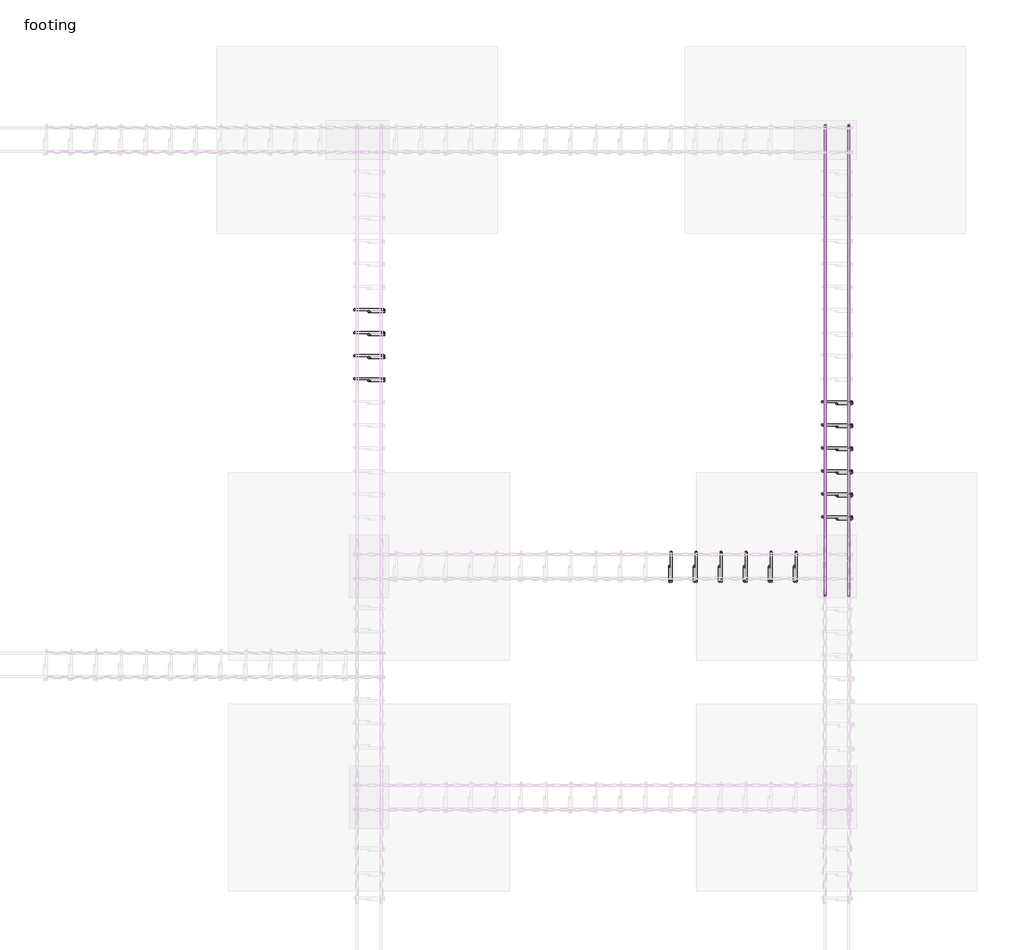
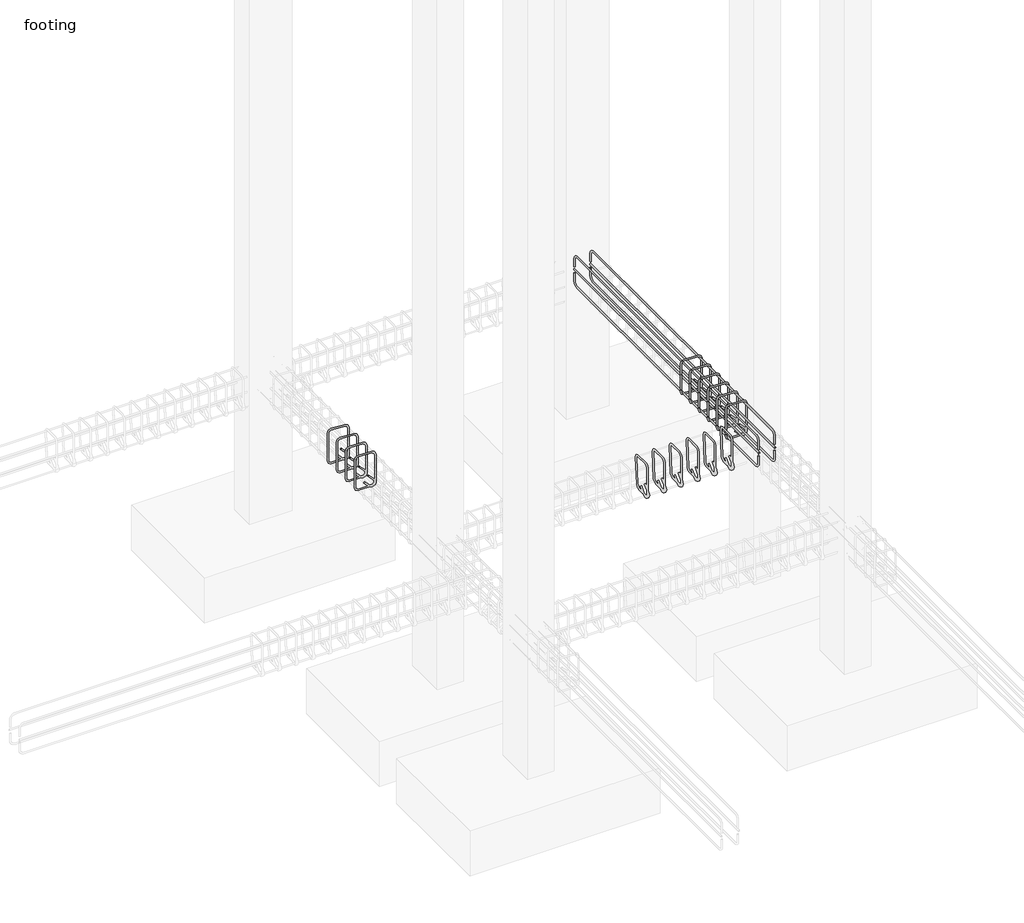
# One storey, part 19 of 21: 23 reinforcing bars.
"""IFC4 building model written with IfcOpenShell, lengths in millimetres."""

from ifc_helpers import new_model, si_unit, point, frame, origin, place, context, project, spatial, polyline, circle_curve, trimmed, segment, composite_curve, element, save
from ifc_brep_helpers import swept_disk

model = new_model("IFC4")

# Units and contexts
model_context = context("Model", 3, world=origin())
ifc_project = project(units=[si_unit("LENGTHUNIT", "METRE", prefix="MILLI")], contexts=[model_context])

# Site, building, storey
site = spatial("IfcSite", under=ifc_project)
building = spatial("IfcBuilding", under=site)
storey = spatial("IfcBuildingStorey", under=building, Name="footing", Elevation=-1524.0)

# Reinforcing bars
placement = place(None, origin())
element("IfcReinforcingBar", 1, at=placement, inside=storey, context=model_context, shape_type="SolidModel", body=[
    swept_disk(composite_curve([segment(polyline([(-5910.0883428, 8213.6387132, -310.8825168), (-5910.0883428, 8158.7737147, -365.7475153)]), True, "CONTINUOUS"), segment(trimmed(circle_curve(frame((-5910.0883428, 8136.3230744, -343.296875), z_axis=(-1.0, 0.0, 0.0), x_axis=(0.0, 22.450640299999577, -22.450640299999975)), 31.75), [point((-5910.0883428, 8158.7737147, -365.7475153))], [point((-5910.0883428, 8104.5730744, -343.296875))], True, "CARTESIAN"), True, "CONTINUOUS"), segment(polyline([(-5910.0883428, 8104.5730744, -343.296875), (-5910.0883428, 8104.5730744, -63.103125)]), True, "CONTINUOUS"), segment(trimmed(circle_curve(frame((-5910.0883428, 8136.3230744, -63.103125), z_axis=(-1.0, 0.0, 0.0), x_axis=(0.0, -31.75, 0.0)), 31.75), [point((-5910.0883428, 8104.5730744, -63.103125))], [point((-5910.0883428, 8136.3230744, -31.353125))], True, "CARTESIAN"), True, "CONTINUOUS"), segment(polyline([(-5910.0883428, 8136.3230744, -31.353125), (-5910.0883428, 8264.1168244, -31.353125)]), True, "CONTINUOUS"), segment(trimmed(circle_curve(frame((-5908.9159328, 8264.1168244, -63.0814712), z_axis=(-0.9993179916193466, 0.0, -0.03692629992126919), x_axis=(-1.1724100000001272, 0.0, 31.728346200000004)), 31.75), [point((-5910.0883428, 8264.1168244, -31.353125))], [point((-5908.9159328, 8295.8668244, -63.0814712))], True, "CARTESIAN"), True, "CONTINUOUS"), segment(polyline([(-5908.9159328, 8295.8668244, -63.0814712), (-5898.5607528, 8295.8668244, -343.3185288)]), True, "CONTINUOUS"), segment(trimmed(circle_curve(frame((-5898.5607528, 8264.1168244, -343.3185288), z_axis=(-0.9993179916193466, 0.0, -0.03692629992126919), x_axis=(0.0, 31.75, 0.0)), 31.75), [point((-5898.5607528, 8295.8668244, -343.3185288))], [point((-5897.3883428, 8264.1168244, -375.046875))], True, "CARTESIAN"), True, "CONTINUOUS"), segment(polyline([(-5897.3883428, 8264.1168244, -375.046875), (-5897.3883428, 8136.3230744, -375.046875)]), True, "CONTINUOUS"), segment(trimmed(circle_curve(frame((-5897.3883428, 8136.3230744, -343.296875), z_axis=(-1.0, 0.0, 0.0), x_axis=(0.0, 0.0, -31.75)), 31.75), [point((-5897.3883428, 8136.3230744, -375.046875))], [point((-5897.3883428, 8113.8724341, -320.8462347))], True, "CARTESIAN"), True, "CONTINUOUS"), segment(polyline([(-5897.3883428, 8113.8724341, -320.8462347), (-5897.3883428, 8168.7374326, -265.9812362)]), True, "CONTINUOUS")], self_intersect=False), 6.35),
])
element("IfcReinforcingBar", 2, at=placement, inside=storey, context=model_context, shape_type="SolidModel", body=[
    swept_disk(composite_curve([segment(polyline([(-5747.3883428, 8213.6387132, -310.8825168), (-5747.3883428, 8158.7737147, -365.7475153)]), True, "CONTINUOUS"), segment(trimmed(circle_curve(frame((-5747.3883428, 8136.3230744, -343.296875), z_axis=(-1.0, 0.0, 0.0), x_axis=(0.0, 22.450640299999577, -22.450640299999975)), 31.75), [point((-5747.3883428, 8158.7737147, -365.7475153))], [point((-5747.3883428, 8104.5730744, -343.296875))], True, "CARTESIAN"), True, "CONTINUOUS"), segment(polyline([(-5747.3883428, 8104.5730744, -343.296875), (-5747.3883428, 8104.5730744, -63.103125)]), True, "CONTINUOUS"), segment(trimmed(circle_curve(frame((-5747.3883428, 8136.3230744, -63.103125), z_axis=(-1.0, 0.0, 0.0), x_axis=(0.0, -31.75, 0.0)), 31.75), [point((-5747.3883428, 8104.5730744, -63.103125))], [point((-5747.3883428, 8136.3230744, -31.353125))], True, "CARTESIAN"), True, "CONTINUOUS"), segment(polyline([(-5747.3883428, 8136.3230744, -31.353125), (-5747.3883428, 8264.1168244, -31.353125)]), True, "CONTINUOUS"), segment(trimmed(circle_curve(frame((-5746.2159328, 8264.1168244, -63.0814712), z_axis=(-0.9993179916193466, 0.0, -0.03692629992126919), x_axis=(-1.1724100000001272, 0.0, 31.728346200000004)), 31.75), [point((-5747.3883428, 8264.1168244, -31.353125))], [point((-5746.2159328, 8295.8668244, -63.0814712))], True, "CARTESIAN"), True, "CONTINUOUS"), segment(polyline([(-5746.2159328, 8295.8668244, -63.0814712), (-5735.8607528, 8295.8668244, -343.3185288)]), True, "CONTINUOUS"), segment(trimmed(circle_curve(frame((-5735.8607528, 8264.1168244, -343.3185288), z_axis=(-0.9993179916193466, 0.0, -0.03692629992126919), x_axis=(0.0, 31.75, 0.0)), 31.75), [point((-5735.8607528, 8295.8668244, -343.3185288))], [point((-5734.6883428, 8264.1168244, -375.046875))], True, "CARTESIAN"), True, "CONTINUOUS"), segment(polyline([(-5734.6883428, 8264.1168244, -375.046875), (-5734.6883428, 8136.3230744, -375.046875)]), True, "CONTINUOUS"), segment(trimmed(circle_curve(frame((-5734.6883428, 8136.3230744, -343.296875), z_axis=(-1.0, 0.0, 0.0), x_axis=(0.0, 0.0, -31.75)), 31.75), [point((-5734.6883428, 8136.3230744, -375.046875))], [point((-5734.6883428, 8113.8724341, -320.8462347))], True, "CARTESIAN"), True, "CONTINUOUS"), segment(polyline([(-5734.6883428, 8113.8724341, -320.8462347), (-5734.6883428, 8168.7374326, -265.9812362)]), True, "CONTINUOUS")], self_intersect=False), 6.35),
])
element("IfcReinforcingBar", 3, at=placement, inside=storey, context=model_context, shape_type="SolidModel", body=[
    swept_disk(composite_curve([segment(polyline([(-5584.6883428, 8213.6387132, -310.8825168), (-5584.6883428, 8158.7737147, -365.7475153)]), True, "CONTINUOUS"), segment(trimmed(circle_curve(frame((-5584.6883428, 8136.3230744, -343.296875), z_axis=(-1.0, 0.0, 0.0), x_axis=(0.0, 22.450640299999577, -22.450640299999975)), 31.75), [point((-5584.6883428, 8158.7737147, -365.7475153))], [point((-5584.6883428, 8104.5730744, -343.296875))], True, "CARTESIAN"), True, "CONTINUOUS"), segment(polyline([(-5584.6883428, 8104.5730744, -343.296875), (-5584.6883428, 8104.5730744, -63.103125)]), True, "CONTINUOUS"), segment(trimmed(circle_curve(frame((-5584.6883428, 8136.3230744, -63.103125), z_axis=(-1.0, 0.0, 0.0), x_axis=(0.0, -31.75, 0.0)), 31.75), [point((-5584.6883428, 8104.5730744, -63.103125))], [point((-5584.6883428, 8136.3230744, -31.353125))], True, "CARTESIAN"), True, "CONTINUOUS"), segment(polyline([(-5584.6883428, 8136.3230744, -31.353125), (-5584.6883428, 8264.1168244, -31.353125)]), True, "CONTINUOUS"), segment(trimmed(circle_curve(frame((-5583.5159328, 8264.1168244, -63.0814712), z_axis=(-0.9993179916193466, 0.0, -0.03692629992126919), x_axis=(-1.1724100000001272, 0.0, 31.728346200000004)), 31.75), [point((-5584.6883428, 8264.1168244, -31.353125))], [point((-5583.5159328, 8295.8668244, -63.0814712))], True, "CARTESIAN"), True, "CONTINUOUS"), segment(polyline([(-5583.5159328, 8295.8668244, -63.0814712), (-5573.1607528, 8295.8668244, -343.3185288)]), True, "CONTINUOUS"), segment(trimmed(circle_curve(frame((-5573.1607528, 8264.1168244, -343.3185288), z_axis=(-0.9993179916193466, 0.0, -0.03692629992126919), x_axis=(0.0, 31.75, 0.0)), 31.75), [point((-5573.1607528, 8295.8668244, -343.3185288))], [point((-5571.9883428, 8264.1168244, -375.046875))], True, "CARTESIAN"), True, "CONTINUOUS"), segment(polyline([(-5571.9883428, 8264.1168244, -375.046875), (-5571.9883428, 8136.3230744, -375.046875)]), True, "CONTINUOUS"), segment(trimmed(circle_curve(frame((-5571.9883428, 8136.3230744, -343.296875), z_axis=(-1.0, 0.0, 0.0), x_axis=(0.0, 0.0, -31.75)), 31.75), [point((-5571.9883428, 8136.3230744, -375.046875))], [point((-5571.9883428, 8113.8724341, -320.8462347))], True, "CARTESIAN"), True, "CONTINUOUS"), segment(polyline([(-5571.9883428, 8113.8724341, -320.8462347), (-5571.9883428, 8168.7374326, -265.9812362)]), True, "CONTINUOUS")], self_intersect=False), 6.35),
])
element("IfcReinforcingBar", 4, at=placement, inside=storey, context=model_context, shape_type="SolidModel", body=[
    swept_disk(composite_curve([segment(polyline([(-5421.9883428, 8213.6387132, -310.8825168), (-5421.9883428, 8158.7737147, -365.7475153)]), True, "CONTINUOUS"), segment(trimmed(circle_curve(frame((-5421.9883428, 8136.3230744, -343.296875), z_axis=(-1.0, 0.0, 0.0), x_axis=(0.0, 22.450640299999577, -22.450640299999975)), 31.75), [point((-5421.9883428, 8158.7737147, -365.7475153))], [point((-5421.9883428, 8104.5730744, -343.296875))], True, "CARTESIAN"), True, "CONTINUOUS"), segment(polyline([(-5421.9883428, 8104.5730744, -343.296875), (-5421.9883428, 8104.5730744, -63.103125)]), True, "CONTINUOUS"), segment(trimmed(circle_curve(frame((-5421.9883428, 8136.3230744, -63.103125), z_axis=(-1.0, 0.0, 0.0), x_axis=(0.0, -31.75, 0.0)), 31.75), [point((-5421.9883428, 8104.5730744, -63.103125))], [point((-5421.9883428, 8136.3230744, -31.353125))], True, "CARTESIAN"), True, "CONTINUOUS"), segment(polyline([(-5421.9883428, 8136.3230744, -31.353125), (-5421.9883428, 8264.1168244, -31.353125)]), True, "CONTINUOUS"), segment(trimmed(circle_curve(frame((-5420.8159328, 8264.1168244, -63.0814712), z_axis=(-0.9993179916193466, 0.0, -0.03692629992126919), x_axis=(-1.1724100000001272, 0.0, 31.728346200000004)), 31.75), [point((-5421.9883428, 8264.1168244, -31.353125))], [point((-5420.8159328, 8295.8668244, -63.0814712))], True, "CARTESIAN"), True, "CONTINUOUS"), segment(polyline([(-5420.8159328, 8295.8668244, -63.0814712), (-5410.4607528, 8295.8668244, -343.3185288)]), True, "CONTINUOUS"), segment(trimmed(circle_curve(frame((-5410.4607528, 8264.1168244, -343.3185288), z_axis=(-0.9993179916193466, 0.0, -0.03692629992126919), x_axis=(0.0, 31.75, 0.0)), 31.75), [point((-5410.4607528, 8295.8668244, -343.3185288))], [point((-5409.2883428, 8264.1168244, -375.046875))], True, "CARTESIAN"), True, "CONTINUOUS"), segment(polyline([(-5409.2883428, 8264.1168244, -375.046875), (-5409.2883428, 8136.3230744, -375.046875)]), True, "CONTINUOUS"), segment(trimmed(circle_curve(frame((-5409.2883428, 8136.3230744, -343.296875), z_axis=(-1.0, 0.0, 0.0), x_axis=(0.0, 0.0, -31.75)), 31.75), [point((-5409.2883428, 8136.3230744, -375.046875))], [point((-5409.2883428, 8113.8724341, -320.8462347))], True, "CARTESIAN"), True, "CONTINUOUS"), segment(polyline([(-5409.2883428, 8113.8724341, -320.8462347), (-5409.2883428, 8168.7374326, -265.9812362)]), True, "CONTINUOUS")], self_intersect=False), 6.35),
])
element("IfcReinforcingBar", 5, at=placement, inside=storey, context=model_context, shape_type="SolidModel", body=[
    swept_disk(composite_curve([segment(polyline([(-5259.2883428, 8213.6387132, -310.8825168), (-5259.2883428, 8158.7737147, -365.7475153)]), True, "CONTINUOUS"), segment(trimmed(circle_curve(frame((-5259.2883428, 8136.3230744, -343.296875), z_axis=(-1.0, 0.0, 0.0), x_axis=(0.0, 22.450640299999577, -22.450640299999975)), 31.75), [point((-5259.2883428, 8158.7737147, -365.7475153))], [point((-5259.2883428, 8104.5730744, -343.296875))], True, "CARTESIAN"), True, "CONTINUOUS"), segment(polyline([(-5259.2883428, 8104.5730744, -343.296875), (-5259.2883428, 8104.5730744, -63.103125)]), True, "CONTINUOUS"), segment(trimmed(circle_curve(frame((-5259.2883428, 8136.3230744, -63.103125), z_axis=(-1.0, 0.0, 0.0), x_axis=(0.0, -31.75, 0.0)), 31.75), [point((-5259.2883428, 8104.5730744, -63.103125))], [point((-5259.2883428, 8136.3230744, -31.353125))], True, "CARTESIAN"), True, "CONTINUOUS"), segment(polyline([(-5259.2883428, 8136.3230744, -31.353125), (-5259.2883428, 8264.1168244, -31.353125)]), True, "CONTINUOUS"), segment(trimmed(circle_curve(frame((-5258.1159328, 8264.1168244, -63.0814712), z_axis=(-0.9993179916193466, 0.0, -0.03692629992126919), x_axis=(-1.1724099999992177, 0.0, 31.728346200000004)), 31.75), [point((-5259.2883428, 8264.1168244, -31.353125))], [point((-5258.1159328, 8295.8668244, -63.0814712))], True, "CARTESIAN"), True, "CONTINUOUS"), segment(polyline([(-5258.1159328, 8295.8668244, -63.0814712), (-5247.7607528, 8295.8668244, -343.3185288)]), True, "CONTINUOUS"), segment(trimmed(circle_curve(frame((-5247.7607528, 8264.1168244, -343.3185288), z_axis=(-0.9993179916193466, 0.0, -0.03692629992126919), x_axis=(0.0, 31.75, 0.0)), 31.75), [point((-5247.7607528, 8295.8668244, -343.3185288))], [point((-5246.5883428, 8264.1168244, -375.046875))], True, "CARTESIAN"), True, "CONTINUOUS"), segment(polyline([(-5246.5883428, 8264.1168244, -375.046875), (-5246.5883428, 8136.3230744, -375.046875)]), True, "CONTINUOUS"), segment(trimmed(circle_curve(frame((-5246.5883428, 8136.3230744, -343.296875), z_axis=(-1.0, 0.0, 0.0), x_axis=(0.0, 0.0, -31.75)), 31.75), [point((-5246.5883428, 8136.3230744, -375.046875))], [point((-5246.5883428, 8113.8724341, -320.8462347))], True, "CARTESIAN"), True, "CONTINUOUS"), segment(polyline([(-5246.5883428, 8113.8724341, -320.8462347), (-5246.5883428, 8168.7374326, -265.9812362)]), True, "CONTINUOUS")], self_intersect=False), 6.35),
])
element("IfcReinforcingBar", 6, at=placement, inside=storey, context=model_context, shape_type="SolidModel", body=[
    swept_disk(composite_curve([segment(polyline([(-5096.5883428, 8213.6387132, -310.8825168), (-5096.5883428, 8158.7737147, -365.7475153)]), True, "CONTINUOUS"), segment(trimmed(circle_curve(frame((-5096.5883428, 8136.3230744, -343.296875), z_axis=(-1.0, 0.0, 0.0), x_axis=(0.0, 22.450640299999577, -22.450640299999975)), 31.75), [point((-5096.5883428, 8158.7737147, -365.7475153))], [point((-5096.5883428, 8104.5730744, -343.296875))], True, "CARTESIAN"), True, "CONTINUOUS"), segment(polyline([(-5096.5883428, 8104.5730744, -343.296875), (-5096.5883428, 8104.5730744, -63.103125)]), True, "CONTINUOUS"), segment(trimmed(circle_curve(frame((-5096.5883428, 8136.3230744, -63.103125), z_axis=(-1.0, 0.0, 0.0), x_axis=(0.0, -31.75, 0.0)), 31.75), [point((-5096.5883428, 8104.5730744, -63.103125))], [point((-5096.5883428, 8136.3230744, -31.353125))], True, "CARTESIAN"), True, "CONTINUOUS"), segment(polyline([(-5096.5883428, 8136.3230744, -31.353125), (-5096.5883428, 8264.1168244, -31.353125)]), True, "CONTINUOUS"), segment(trimmed(circle_curve(frame((-5095.4159328, 8264.1168244, -63.0814712), z_axis=(-0.9993179916193466, 0.0, -0.03692629992126919), x_axis=(-1.1724100000001272, 0.0, 31.728346200000004)), 31.75), [point((-5096.5883428, 8264.1168244, -31.353125))], [point((-5095.4159328, 8295.8668244, -63.0814712))], True, "CARTESIAN"), True, "CONTINUOUS"), segment(polyline([(-5095.4159328, 8295.8668244, -63.0814712), (-5085.0607528, 8295.8668244, -343.3185288)]), True, "CONTINUOUS"), segment(trimmed(circle_curve(frame((-5085.0607528, 8264.1168244, -343.3185288), z_axis=(-0.9993179916193466, 0.0, -0.03692629992126919), x_axis=(0.0, 31.75, 0.0)), 31.75), [point((-5085.0607528, 8295.8668244, -343.3185288))], [point((-5083.8883428, 8264.1168244, -375.046875))], True, "CARTESIAN"), True, "CONTINUOUS"), segment(polyline([(-5083.8883428, 8264.1168244, -375.046875), (-5083.8883428, 8136.3230744, -375.046875)]), True, "CONTINUOUS"), segment(trimmed(circle_curve(frame((-5083.8883428, 8136.3230744, -343.296875), z_axis=(-1.0, 0.0, 0.0), x_axis=(0.0, 0.0, -31.75)), 31.75), [point((-5083.8883428, 8136.3230744, -375.046875))], [point((-5083.8883428, 8113.8724341, -320.8462347))], True, "CARTESIAN"), True, "CONTINUOUS"), segment(polyline([(-5083.8883428, 8113.8724341, -320.8462347), (-5083.8883428, 8168.7374326, -265.9812362)]), True, "CONTINUOUS")], self_intersect=False), 6.35),
])
element("IfcReinforcingBar", 7, at=placement, inside=storey, context=model_context, shape_type="SolidModel", body=[
    swept_disk(composite_curve([segment(polyline([(-7834.7165254, 9425.2699494, -265.9812362), (-7779.851527, 9425.2699494, -320.8462347)]), True, "CONTINUOUS"), segment(trimmed(circle_curve(frame((-7802.3021673, 9425.2699494, -343.296875), z_axis=(0.0, 1.0, 0.0), x_axis=(22.450640300000487, 0.0, 22.450640299999975)), 31.75), [point((-7779.851527, 9425.2699494, -320.8462347))], [point((-7802.3021673, 9425.2699494, -375.046875))], True, "CARTESIAN"), True, "CONTINUOUS"), segment(polyline([(-7802.3021673, 9425.2699494, -375.046875), (-7930.0959173, 9425.2699494, -375.046875)]), True, "CONTINUOUS"), segment(trimmed(circle_curve(frame((-7930.0959173, 9425.2699494, -343.296875), z_axis=(0.0, 1.0, 0.0), x_axis=(0.0, 0.0, -31.75)), 31.75), [point((-7930.0959173, 9425.2699494, -375.046875))], [point((-7961.8459173, 9425.2699494, -343.296875))], True, "CARTESIAN"), True, "CONTINUOUS"), segment(polyline([(-7961.8459173, 9425.2699494, -343.296875), (-7961.8459173, 9425.2699494, -63.103125)]), True, "CONTINUOUS"), segment(trimmed(circle_curve(frame((-7930.165658, 9423.1666957, -63.103125), z_axis=(0.06624421176864137, 0.9978034397651431, 0.0), x_axis=(-31.680259300000216, 2.103253700001005, 0.0)), 31.75), [point((-7961.8459173, 9425.2699494, -63.103125))], [point((-7930.165658, 9423.1666957, -31.353125))], True, "CARTESIAN"), True, "CONTINUOUS"), segment(polyline([(-7930.165658, 9423.1666957, -31.353125), (-7802.2324265, 9414.6732031, -31.353125)]), True, "CONTINUOUS"), segment(trimmed(circle_curve(frame((-7802.2324265, 9414.6732031, -63.103125), z_axis=(0.06624421176864137, 0.9978034397651431, 0.0), x_axis=(0.0, 0.0, 31.75)), 31.75), [point((-7802.2324265, 9414.6732031, -31.353125))], [point((-7770.5521673, 9412.5699494, -63.103125))], True, "CARTESIAN"), True, "CONTINUOUS"), segment(polyline([(-7770.5521673, 9412.5699494, -63.103125), (-7770.5521673, 9412.5699494, -343.296875)]), True, "CONTINUOUS"), segment(trimmed(circle_curve(frame((-7802.3021673, 9412.5699494, -343.296875), z_axis=(0.0, 1.0, 0.0), x_axis=(31.75, 0.0, 0.0)), 31.75), [point((-7770.5521673, 9412.5699494, -343.296875))], [point((-7824.7528076, 9412.5699494, -365.7475153))], True, "CARTESIAN"), True, "CONTINUOUS"), segment(polyline([(-7824.7528076, 9412.5699494, -365.7475153), (-7879.617806, 9412.5699494, -310.8825168)]), True, "CONTINUOUS")], self_intersect=False), 6.35),
])
element("IfcReinforcingBar", 8, at=placement, inside=storey, context=model_context, shape_type="SolidModel", body=[
    swept_disk(composite_curve([segment(polyline([(-7834.7165254, 9575.2699494, -265.9812362), (-7779.851527, 9575.2699494, -320.8462347)]), True, "CONTINUOUS"), segment(trimmed(circle_curve(frame((-7802.3021673, 9575.2699494, -343.296875), z_axis=(0.0, 1.0, 0.0), x_axis=(22.450640300000487, 0.0, 22.450640299999975)), 31.75), [point((-7779.851527, 9575.2699494, -320.8462347))], [point((-7802.3021673, 9575.2699494, -375.046875))], True, "CARTESIAN"), True, "CONTINUOUS"), segment(polyline([(-7802.3021673, 9575.2699494, -375.046875), (-7930.0959173, 9575.2699494, -375.046875)]), True, "CONTINUOUS"), segment(trimmed(circle_curve(frame((-7930.0959173, 9575.2699494, -343.296875), z_axis=(0.0, 1.0, 0.0), x_axis=(0.0, 0.0, -31.75)), 31.75), [point((-7930.0959173, 9575.2699494, -375.046875))], [point((-7961.8459173, 9575.2699494, -343.296875))], True, "CARTESIAN"), True, "CONTINUOUS"), segment(polyline([(-7961.8459173, 9575.2699494, -343.296875), (-7961.8459173, 9575.2699494, -63.103125)]), True, "CONTINUOUS"), segment(trimmed(circle_curve(frame((-7930.165658, 9573.1666957, -63.103125), z_axis=(0.06624421176864137, 0.9978034397651431, 0.0), x_axis=(-31.680259300000216, 2.103253700001005, 0.0)), 31.75), [point((-7961.8459173, 9575.2699494, -63.103125))], [point((-7930.165658, 9573.1666957, -31.353125))], True, "CARTESIAN"), True, "CONTINUOUS"), segment(polyline([(-7930.165658, 9573.1666957, -31.353125), (-7802.2324265, 9564.6732031, -31.353125)]), True, "CONTINUOUS"), segment(trimmed(circle_curve(frame((-7802.2324265, 9564.6732031, -63.103125), z_axis=(0.06624421176864137, 0.9978034397651431, 0.0), x_axis=(0.0, 0.0, 31.75)), 31.75), [point((-7802.2324265, 9564.6732031, -31.353125))], [point((-7770.5521673, 9562.5699494, -63.103125))], True, "CARTESIAN"), True, "CONTINUOUS"), segment(polyline([(-7770.5521673, 9562.5699494, -63.103125), (-7770.5521673, 9562.5699494, -343.296875)]), True, "CONTINUOUS"), segment(trimmed(circle_curve(frame((-7802.3021673, 9562.5699494, -343.296875), z_axis=(0.0, 1.0, 0.0), x_axis=(31.75, 0.0, 0.0)), 31.75), [point((-7770.5521673, 9562.5699494, -343.296875))], [point((-7824.7528076, 9562.5699494, -365.7475153))], True, "CARTESIAN"), True, "CONTINUOUS"), segment(polyline([(-7824.7528076, 9562.5699494, -365.7475153), (-7879.617806, 9562.5699494, -310.8825168)]), True, "CONTINUOUS")], self_intersect=False), 6.35),
])
element("IfcReinforcingBar", 9, at=placement, inside=storey, context=model_context, shape_type="SolidModel", body=[
    swept_disk(composite_curve([segment(polyline([(-7834.7165254, 9725.2699494, -265.9812362), (-7779.851527, 9725.2699494, -320.8462347)]), True, "CONTINUOUS"), segment(trimmed(circle_curve(frame((-7802.3021673, 9725.2699494, -343.296875), z_axis=(0.0, 1.0, 0.0), x_axis=(22.450640300000487, 0.0, 22.450640299999975)), 31.75), [point((-7779.851527, 9725.2699494, -320.8462347))], [point((-7802.3021673, 9725.2699494, -375.046875))], True, "CARTESIAN"), True, "CONTINUOUS"), segment(polyline([(-7802.3021673, 9725.2699494, -375.046875), (-7930.0959173, 9725.2699494, -375.046875)]), True, "CONTINUOUS"), segment(trimmed(circle_curve(frame((-7930.0959173, 9725.2699494, -343.296875), z_axis=(0.0, 1.0, 0.0), x_axis=(0.0, 0.0, -31.75)), 31.75), [point((-7930.0959173, 9725.2699494, -375.046875))], [point((-7961.8459173, 9725.2699494, -343.296875))], True, "CARTESIAN"), True, "CONTINUOUS"), segment(polyline([(-7961.8459173, 9725.2699494, -343.296875), (-7961.8459173, 9725.2699494, -63.103125)]), True, "CONTINUOUS"), segment(trimmed(circle_curve(frame((-7930.165658, 9723.1666957, -63.103125), z_axis=(0.06624421176864137, 0.9978034397651431, 0.0), x_axis=(-31.680259300000216, 2.103253700001005, 0.0)), 31.75), [point((-7961.8459173, 9725.2699494, -63.103125))], [point((-7930.165658, 9723.1666957, -31.353125))], True, "CARTESIAN"), True, "CONTINUOUS"), segment(polyline([(-7930.165658, 9723.1666957, -31.353125), (-7802.2324265, 9714.6732031, -31.353125)]), True, "CONTINUOUS"), segment(trimmed(circle_curve(frame((-7802.2324265, 9714.6732031, -63.103125), z_axis=(0.06624421176864137, 0.9978034397651431, 0.0), x_axis=(0.0, 0.0, 31.75)), 31.75), [point((-7802.2324265, 9714.6732031, -31.353125))], [point((-7770.5521673, 9712.5699494, -63.103125))], True, "CARTESIAN"), True, "CONTINUOUS"), segment(polyline([(-7770.5521673, 9712.5699494, -63.103125), (-7770.5521673, 9712.5699494, -343.296875)]), True, "CONTINUOUS"), segment(trimmed(circle_curve(frame((-7802.3021673, 9712.5699494, -343.296875), z_axis=(0.0, 1.0, 0.0), x_axis=(31.75, 0.0, 0.0)), 31.75), [point((-7770.5521673, 9712.5699494, -343.296875))], [point((-7824.7528076, 9712.5699494, -365.7475153))], True, "CARTESIAN"), True, "CONTINUOUS"), segment(polyline([(-7824.7528076, 9712.5699494, -365.7475153), (-7879.617806, 9712.5699494, -310.8825168)]), True, "CONTINUOUS")], self_intersect=False), 6.35),
])
element("IfcReinforcingBar", 10, at=placement, inside=storey, context=model_context, shape_type="SolidModel", body=[
    swept_disk(composite_curve([segment(polyline([(-7834.7165254, 9875.2699494, -265.9812362), (-7779.851527, 9875.2699494, -320.8462347)]), True, "CONTINUOUS"), segment(trimmed(circle_curve(frame((-7802.3021673, 9875.2699494, -343.296875), z_axis=(0.0, 1.0, 0.0), x_axis=(22.450640300000487, 0.0, 22.450640299999975)), 31.75), [point((-7779.851527, 9875.2699494, -320.8462347))], [point((-7802.3021673, 9875.2699494, -375.046875))], True, "CARTESIAN"), True, "CONTINUOUS"), segment(polyline([(-7802.3021673, 9875.2699494, -375.046875), (-7930.0959173, 9875.2699494, -375.046875)]), True, "CONTINUOUS"), segment(trimmed(circle_curve(frame((-7930.0959173, 9875.2699494, -343.296875), z_axis=(0.0, 1.0, 0.0), x_axis=(0.0, 0.0, -31.75)), 31.75), [point((-7930.0959173, 9875.2699494, -375.046875))], [point((-7961.8459173, 9875.2699494, -343.296875))], True, "CARTESIAN"), True, "CONTINUOUS"), segment(polyline([(-7961.8459173, 9875.2699494, -343.296875), (-7961.8459173, 9875.2699494, -63.103125)]), True, "CONTINUOUS"), segment(trimmed(circle_curve(frame((-7930.165658, 9873.1666957, -63.103125), z_axis=(0.06624421176864137, 0.9978034397651431, 0.0), x_axis=(-31.680259300000216, 2.103253700001005, 0.0)), 31.75), [point((-7961.8459173, 9875.2699494, -63.103125))], [point((-7930.165658, 9873.1666957, -31.353125))], True, "CARTESIAN"), True, "CONTINUOUS"), segment(polyline([(-7930.165658, 9873.1666957, -31.353125), (-7802.2324265, 9864.6732031, -31.353125)]), True, "CONTINUOUS"), segment(trimmed(circle_curve(frame((-7802.2324265, 9864.6732031, -63.103125), z_axis=(0.06624421176864137, 0.9978034397651431, 0.0), x_axis=(0.0, 0.0, 31.75)), 31.75), [point((-7802.2324265, 9864.6732031, -31.353125))], [point((-7770.5521673, 9862.5699494, -63.103125))], True, "CARTESIAN"), True, "CONTINUOUS"), segment(polyline([(-7770.5521673, 9862.5699494, -63.103125), (-7770.5521673, 9862.5699494, -343.296875)]), True, "CONTINUOUS"), segment(trimmed(circle_curve(frame((-7802.3021673, 9862.5699494, -343.296875), z_axis=(0.0, 1.0, 0.0), x_axis=(31.75, 0.0, 0.0)), 31.75), [point((-7770.5521673, 9862.5699494, -343.296875))], [point((-7824.7528076, 9862.5699494, -365.7475153))], True, "CARTESIAN"), True, "CONTINUOUS"), segment(polyline([(-7824.7528076, 9862.5699494, -365.7475153), (-7879.617806, 9862.5699494, -310.8825168)]), True, "CONTINUOUS")], self_intersect=False), 6.35),
])
element("IfcReinforcingBar", 11, at=placement, inside=storey, context=model_context, shape_type="SolidModel", body=[
    swept_disk(composite_curve([segment(polyline([(-4786.7165254, 8525.2699494, -265.9812362), (-4731.851527, 8525.2699494, -320.8462347)]), True, "CONTINUOUS"), segment(trimmed(circle_curve(frame((-4754.3021673, 8525.2699494, -343.296875), z_axis=(0.0, 1.0, 0.0), x_axis=(22.450640300000487, 0.0, 22.450640299999975)), 31.75), [point((-4731.851527, 8525.2699494, -320.8462347))], [point((-4754.3021673, 8525.2699494, -375.046875))], True, "CARTESIAN"), True, "CONTINUOUS"), segment(polyline([(-4754.3021673, 8525.2699494, -375.046875), (-4882.0959173, 8525.2699494, -375.046875)]), True, "CONTINUOUS"), segment(trimmed(circle_curve(frame((-4882.0959173, 8525.2699494, -343.296875), z_axis=(0.0, 1.0, 0.0), x_axis=(0.0, 0.0, -31.75)), 31.75), [point((-4882.0959173, 8525.2699494, -375.046875))], [point((-4913.8459173, 8525.2699494, -343.296875))], True, "CARTESIAN"), True, "CONTINUOUS"), segment(polyline([(-4913.8459173, 8525.2699494, -343.296875), (-4913.8459173, 8525.2699494, -63.103125)]), True, "CONTINUOUS"), segment(trimmed(circle_curve(frame((-4882.165658, 8523.1666957, -63.103125), z_axis=(0.06624421176864137, 0.9978034397651431, 0.0), x_axis=(-31.680259300000216, 2.103253700001005, 0.0)), 31.75), [point((-4913.8459173, 8525.2699494, -63.103125))], [point((-4882.165658, 8523.1666957, -31.353125))], True, "CARTESIAN"), True, "CONTINUOUS"), segment(polyline([(-4882.165658, 8523.1666957, -31.353125), (-4754.2324265, 8514.6732031, -31.353125)]), True, "CONTINUOUS"), segment(trimmed(circle_curve(frame((-4754.2324265, 8514.6732031, -63.103125), z_axis=(0.06624421176864137, 0.9978034397651431, 0.0), x_axis=(0.0, 0.0, 31.75)), 31.75), [point((-4754.2324265, 8514.6732031, -31.353125))], [point((-4722.5521673, 8512.5699494, -63.103125))], True, "CARTESIAN"), True, "CONTINUOUS"), segment(polyline([(-4722.5521673, 8512.5699494, -63.103125), (-4722.5521673, 8512.5699494, -343.296875)]), True, "CONTINUOUS"), segment(trimmed(circle_curve(frame((-4754.3021673, 8512.5699494, -343.296875), z_axis=(0.0, 1.0, 0.0), x_axis=(31.75, 0.0, 0.0)), 31.75), [point((-4722.5521673, 8512.5699494, -343.296875))], [point((-4776.7528076, 8512.5699494, -365.7475153))], True, "CARTESIAN"), True, "CONTINUOUS"), segment(polyline([(-4776.7528076, 8512.5699494, -365.7475153), (-4831.617806, 8512.5699494, -310.8825168)]), True, "CONTINUOUS")], self_intersect=False), 6.35),
])
element("IfcReinforcingBar", 12, at=placement, inside=storey, context=model_context, shape_type="SolidModel", body=[
    swept_disk(composite_curve([segment(polyline([(-4740.8317831, 8012.5359344, -170.2827408), (-4740.8317831, 8012.5359344, -94.0827408)]), True, "CONTINUOUS"), segment(trimmed(circle_curve(frame((-4740.8317831, 8056.9859344, -94.0827408), z_axis=(-1.0, 0.0, 0.0), x_axis=(0.0, -44.44999999999982, 0.0)), 44.45), [point((-4740.8317831, 8012.5359344, -94.0827408))], [point((-4740.8317831, 8056.9859344, -49.6327408))], True, "CARTESIAN"), True, "CONTINUOUS"), segment(polyline([(-4740.8317831, 8056.9859344, -49.6327408), (-4740.8317831, 11032.7168244, -49.6327408)]), True, "CONTINUOUS"), segment(trimmed(circle_curve(frame((-4740.8317831, 11032.7168244, -94.0827408), z_axis=(-1.0, 0.0, 0.0), x_axis=(0.0, 0.0, 44.449999999999996)), 44.45), [point((-4740.8317831, 11032.7168244, -49.6327408))], [point((-4740.8317831, 11077.1668244, -94.0827408))], True, "CARTESIAN"), True, "CONTINUOUS"), segment(polyline([(-4740.8317831, 11077.1668244, -94.0827408), (-4740.8317831, 11077.1668244, -170.2827408)]), True, "CONTINUOUS")], self_intersect=False), 6.35),
])
element("IfcReinforcingBar", 13, at=placement, inside=storey, context=model_context, shape_type="SolidModel", body=[
    swept_disk(composite_curve([segment(polyline([(-4895.5663014, 8012.5359344, -170.2827408), (-4895.5663014, 8012.5359344, -94.0827408)]), True, "CONTINUOUS"), segment(trimmed(circle_curve(frame((-4895.5663014, 8056.9859344, -94.0827408), z_axis=(-1.0, 0.0, 0.0), x_axis=(0.0, -44.44999999999982, 0.0)), 44.45), [point((-4895.5663014, 8012.5359344, -94.0827408))], [point((-4895.5663014, 8056.9859344, -49.6327408))], True, "CARTESIAN"), True, "CONTINUOUS"), segment(polyline([(-4895.5663014, 8056.9859344, -49.6327408), (-4895.5663014, 11032.7168244, -49.6327408)]), True, "CONTINUOUS"), segment(trimmed(circle_curve(frame((-4895.5663014, 11032.7168244, -94.0827408), z_axis=(-1.0, 0.0, 0.0), x_axis=(0.0, 0.0, 44.449999999999996)), 44.45), [point((-4895.5663014, 11032.7168244, -49.6327408))], [point((-4895.5663014, 11077.1668244, -94.0827408))], True, "CARTESIAN"), True, "CONTINUOUS"), segment(polyline([(-4895.5663014, 11077.1668244, -94.0827408), (-4895.5663014, 11077.1668244, -170.2827408)]), True, "CONTINUOUS")], self_intersect=False), 6.35),
])
element("IfcReinforcingBar", 14, at=placement, inside=storey, context=model_context, shape_type="SolidModel", body=[
    swept_disk(composite_curve([segment(polyline([(-4740.8317831, 8012.5359344, -236.1172592), (-4740.8317831, 8012.5359344, -312.3172592)]), True, "CONTINUOUS"), segment(trimmed(circle_curve(frame((-4740.8317831, 8056.9859344, -312.3172592), z_axis=(1.0, 0.0, 0.0), x_axis=(0.0, -44.44999999999982, 0.0)), 44.45), [point((-4740.8317831, 8012.5359344, -312.3172592))], [point((-4740.8317831, 8056.9859344, -356.7672592))], True, "CARTESIAN"), True, "CONTINUOUS"), segment(polyline([(-4740.8317831, 8056.9859344, -356.7672592), (-4740.8317831, 11032.7168244, -356.7672592)]), True, "CONTINUOUS"), segment(trimmed(circle_curve(frame((-4740.8317831, 11032.7168244, -312.3172592), z_axis=(1.0, 0.0, 0.0), x_axis=(0.0, 0.0, -44.44999999999999)), 44.45), [point((-4740.8317831, 11032.7168244, -356.7672592))], [point((-4740.8317831, 11077.1668244, -312.3172592))], True, "CARTESIAN"), True, "CONTINUOUS"), segment(polyline([(-4740.8317831, 11077.1668244, -312.3172592), (-4740.8317831, 11077.1668244, -236.1172592)]), True, "CONTINUOUS")], self_intersect=False), 6.35),
])
element("IfcReinforcingBar", 15, at=placement, inside=storey, context=model_context, shape_type="SolidModel", body=[
    swept_disk(composite_curve([segment(polyline([(-4895.5663014, 8012.5359344, -236.1172592), (-4895.5663014, 8012.5359344, -312.3172592)]), True, "CONTINUOUS"), segment(trimmed(circle_curve(frame((-4895.5663014, 8056.9859344, -312.3172592), z_axis=(1.0, 0.0, 0.0), x_axis=(0.0, -44.44999999999982, 0.0)), 44.45), [point((-4895.5663014, 8012.5359344, -312.3172592))], [point((-4895.5663014, 8056.9859344, -356.7672592))], True, "CARTESIAN"), True, "CONTINUOUS"), segment(polyline([(-4895.5663014, 8056.9859344, -356.7672592), (-4895.5663014, 11032.7168244, -356.7672592)]), True, "CONTINUOUS"), segment(trimmed(circle_curve(frame((-4895.5663014, 11032.7168244, -312.3172592), z_axis=(1.0, 0.0, 0.0), x_axis=(0.0, 0.0, -44.44999999999999)), 44.45), [point((-4895.5663014, 11032.7168244, -356.7672592))], [point((-4895.5663014, 11077.1668244, -312.3172592))], True, "CARTESIAN"), True, "CONTINUOUS"), segment(polyline([(-4895.5663014, 11077.1668244, -312.3172592), (-4895.5663014, 11077.1668244, -236.1172592)]), True, "CONTINUOUS")], self_intersect=False), 6.35),
])
element("IfcReinforcingBar", 16, at=placement, inside=storey, context=model_context, shape_type="SolidModel", body=[
    swept_disk(composite_curve([segment(polyline([(-4895.5663014, 8006.1859344, -203.2), (-4895.5663014, 11083.5168244, -203.2)]), True, "CONTINUOUS")], self_intersect=False), 6.35),
])
element("IfcReinforcingBar", 17, at=placement, inside=storey, context=model_context, shape_type="SolidModel", body=[
    swept_disk(composite_curve([segment(polyline([(-4895.5663014, 8006.1859344, -203.2), (-4895.5663014, 11083.5168244, -203.2)]), True, "CONTINUOUS")], self_intersect=False), 6.35),
])
element("IfcReinforcingBar", 18, at=placement, inside=storey, context=model_context, shape_type="SolidModel", body=[
    swept_disk(composite_curve([segment(polyline([(-4740.8317831, 8006.1859344, -203.2), (-4740.8317831, 11083.5168244, -203.2)]), True, "CONTINUOUS")], self_intersect=False), 6.35),
])
element("IfcReinforcingBar", 19, at=placement, inside=storey, context=model_context, shape_type="SolidModel", body=[
    swept_disk(composite_curve([segment(polyline([(-4786.7165254, 8675.2699494, -265.9812362), (-4731.851527, 8675.2699494, -320.8462347)]), True, "CONTINUOUS"), segment(trimmed(circle_curve(frame((-4754.3021673, 8675.2699494, -343.296875), z_axis=(0.0, 1.0, 0.0), x_axis=(22.450640300000487, 0.0, 22.450640299999975)), 31.75), [point((-4731.851527, 8675.2699494, -320.8462347))], [point((-4754.3021673, 8675.2699494, -375.046875))], True, "CARTESIAN"), True, "CONTINUOUS"), segment(polyline([(-4754.3021673, 8675.2699494, -375.046875), (-4882.0959173, 8675.2699494, -375.046875)]), True, "CONTINUOUS"), segment(trimmed(circle_curve(frame((-4882.0959173, 8675.2699494, -343.296875), z_axis=(0.0, 1.0, 0.0), x_axis=(0.0, 0.0, -31.75)), 31.75), [point((-4882.0959173, 8675.2699494, -375.046875))], [point((-4913.8459173, 8675.2699494, -343.296875))], True, "CARTESIAN"), True, "CONTINUOUS"), segment(polyline([(-4913.8459173, 8675.2699494, -343.296875), (-4913.8459173, 8675.2699494, -63.103125)]), True, "CONTINUOUS"), segment(trimmed(circle_curve(frame((-4882.165658, 8673.1666957, -63.103125), z_axis=(0.06624421176864137, 0.9978034397651431, 0.0), x_axis=(-31.680259300000216, 2.103253700001005, 0.0)), 31.75), [point((-4913.8459173, 8675.2699494, -63.103125))], [point((-4882.165658, 8673.1666957, -31.353125))], True, "CARTESIAN"), True, "CONTINUOUS"), segment(polyline([(-4882.165658, 8673.1666957, -31.353125), (-4754.2324265, 8664.6732031, -31.353125)]), True, "CONTINUOUS"), segment(trimmed(circle_curve(frame((-4754.2324265, 8664.6732031, -63.103125), z_axis=(0.06624421176864137, 0.9978034397651431, 0.0), x_axis=(0.0, 0.0, 31.75)), 31.75), [point((-4754.2324265, 8664.6732031, -31.353125))], [point((-4722.5521673, 8662.5699494, -63.103125))], True, "CARTESIAN"), True, "CONTINUOUS"), segment(polyline([(-4722.5521673, 8662.5699494, -63.103125), (-4722.5521673, 8662.5699494, -343.296875)]), True, "CONTINUOUS"), segment(trimmed(circle_curve(frame((-4754.3021673, 8662.5699494, -343.296875), z_axis=(0.0, 1.0, 0.0), x_axis=(31.75, 0.0, 0.0)), 31.75), [point((-4722.5521673, 8662.5699494, -343.296875))], [point((-4776.7528076, 8662.5699494, -365.7475153))], True, "CARTESIAN"), True, "CONTINUOUS"), segment(polyline([(-4776.7528076, 8662.5699494, -365.7475153), (-4831.617806, 8662.5699494, -310.8825168)]), True, "CONTINUOUS")], self_intersect=False), 6.35),
])
element("IfcReinforcingBar", 20, at=placement, inside=storey, context=model_context, shape_type="SolidModel", body=[
    swept_disk(composite_curve([segment(polyline([(-4786.7165254, 8825.2699494, -265.9812362), (-4731.851527, 8825.2699494, -320.8462347)]), True, "CONTINUOUS"), segment(trimmed(circle_curve(frame((-4754.3021673, 8825.2699494, -343.296875), z_axis=(0.0, 1.0, 0.0), x_axis=(22.450640300000487, 0.0, 22.450640299999975)), 31.75), [point((-4731.851527, 8825.2699494, -320.8462347))], [point((-4754.3021673, 8825.2699494, -375.046875))], True, "CARTESIAN"), True, "CONTINUOUS"), segment(polyline([(-4754.3021673, 8825.2699494, -375.046875), (-4882.0959173, 8825.2699494, -375.046875)]), True, "CONTINUOUS"), segment(trimmed(circle_curve(frame((-4882.0959173, 8825.2699494, -343.296875), z_axis=(0.0, 1.0, 0.0), x_axis=(0.0, 0.0, -31.75)), 31.75), [point((-4882.0959173, 8825.2699494, -375.046875))], [point((-4913.8459173, 8825.2699494, -343.296875))], True, "CARTESIAN"), True, "CONTINUOUS"), segment(polyline([(-4913.8459173, 8825.2699494, -343.296875), (-4913.8459173, 8825.2699494, -63.103125)]), True, "CONTINUOUS"), segment(trimmed(circle_curve(frame((-4882.165658, 8823.1666957, -63.103125), z_axis=(0.06624421176864137, 0.9978034397651431, 0.0), x_axis=(-31.680259300000216, 2.103253700001005, 0.0)), 31.75), [point((-4913.8459173, 8825.2699494, -63.103125))], [point((-4882.165658, 8823.1666957, -31.353125))], True, "CARTESIAN"), True, "CONTINUOUS"), segment(polyline([(-4882.165658, 8823.1666957, -31.353125), (-4754.2324265, 8814.6732031, -31.353125)]), True, "CONTINUOUS"), segment(trimmed(circle_curve(frame((-4754.2324265, 8814.6732031, -63.103125), z_axis=(0.06624421176864137, 0.9978034397651431, 0.0), x_axis=(0.0, 0.0, 31.75)), 31.75), [point((-4754.2324265, 8814.6732031, -31.353125))], [point((-4722.5521673, 8812.5699494, -63.103125))], True, "CARTESIAN"), True, "CONTINUOUS"), segment(polyline([(-4722.5521673, 8812.5699494, -63.103125), (-4722.5521673, 8812.5699494, -343.296875)]), True, "CONTINUOUS"), segment(trimmed(circle_curve(frame((-4754.3021673, 8812.5699494, -343.296875), z_axis=(0.0, 1.0, 0.0), x_axis=(31.75, 0.0, 0.0)), 31.75), [point((-4722.5521673, 8812.5699494, -343.296875))], [point((-4776.7528076, 8812.5699494, -365.7475153))], True, "CARTESIAN"), True, "CONTINUOUS"), segment(polyline([(-4776.7528076, 8812.5699494, -365.7475153), (-4831.617806, 8812.5699494, -310.8825168)]), True, "CONTINUOUS")], self_intersect=False), 6.35),
])
element("IfcReinforcingBar", 21, at=placement, inside=storey, context=model_context, shape_type="SolidModel", body=[
    swept_disk(composite_curve([segment(polyline([(-4786.7165254, 8975.2699494, -265.9812362), (-4731.851527, 8975.2699494, -320.8462347)]), True, "CONTINUOUS"), segment(trimmed(circle_curve(frame((-4754.3021673, 8975.2699494, -343.296875), z_axis=(0.0, 1.0, 0.0), x_axis=(22.450640300000487, 0.0, 22.450640299999975)), 31.75), [point((-4731.851527, 8975.2699494, -320.8462347))], [point((-4754.3021673, 8975.2699494, -375.046875))], True, "CARTESIAN"), True, "CONTINUOUS"), segment(polyline([(-4754.3021673, 8975.2699494, -375.046875), (-4882.0959173, 8975.2699494, -375.046875)]), True, "CONTINUOUS"), segment(trimmed(circle_curve(frame((-4882.0959173, 8975.2699494, -343.296875), z_axis=(0.0, 1.0, 0.0), x_axis=(0.0, 0.0, -31.75)), 31.75), [point((-4882.0959173, 8975.2699494, -375.046875))], [point((-4913.8459173, 8975.2699494, -343.296875))], True, "CARTESIAN"), True, "CONTINUOUS"), segment(polyline([(-4913.8459173, 8975.2699494, -343.296875), (-4913.8459173, 8975.2699494, -63.103125)]), True, "CONTINUOUS"), segment(trimmed(circle_curve(frame((-4882.165658, 8973.1666957, -63.103125), z_axis=(0.06624421176864137, 0.9978034397651431, 0.0), x_axis=(-31.680259300000216, 2.103253700001005, 0.0)), 31.75), [point((-4913.8459173, 8975.2699494, -63.103125))], [point((-4882.165658, 8973.1666957, -31.353125))], True, "CARTESIAN"), True, "CONTINUOUS"), segment(polyline([(-4882.165658, 8973.1666957, -31.353125), (-4754.2324265, 8964.6732031, -31.353125)]), True, "CONTINUOUS"), segment(trimmed(circle_curve(frame((-4754.2324265, 8964.6732031, -63.103125), z_axis=(0.06624421176864137, 0.9978034397651431, 0.0), x_axis=(0.0, 0.0, 31.75)), 31.75), [point((-4754.2324265, 8964.6732031, -31.353125))], [point((-4722.5521673, 8962.5699494, -63.103125))], True, "CARTESIAN"), True, "CONTINUOUS"), segment(polyline([(-4722.5521673, 8962.5699494, -63.103125), (-4722.5521673, 8962.5699494, -343.296875)]), True, "CONTINUOUS"), segment(trimmed(circle_curve(frame((-4754.3021673, 8962.5699494, -343.296875), z_axis=(0.0, 1.0, 0.0), x_axis=(31.75, 0.0, 0.0)), 31.75), [point((-4722.5521673, 8962.5699494, -343.296875))], [point((-4776.7528076, 8962.5699494, -365.7475153))], True, "CARTESIAN"), True, "CONTINUOUS"), segment(polyline([(-4776.7528076, 8962.5699494, -365.7475153), (-4831.617806, 8962.5699494, -310.8825168)]), True, "CONTINUOUS")], self_intersect=False), 6.35),
])
element("IfcReinforcingBar", 22, at=placement, inside=storey, context=model_context, shape_type="SolidModel", body=[
    swept_disk(composite_curve([segment(polyline([(-4786.7165254, 9125.2699494, -265.9812362), (-4731.851527, 9125.2699494, -320.8462347)]), True, "CONTINUOUS"), segment(trimmed(circle_curve(frame((-4754.3021673, 9125.2699494, -343.296875), z_axis=(0.0, 1.0, 0.0), x_axis=(22.450640300000487, 0.0, 22.450640299999975)), 31.75), [point((-4731.851527, 9125.2699494, -320.8462347))], [point((-4754.3021673, 9125.2699494, -375.046875))], True, "CARTESIAN"), True, "CONTINUOUS"), segment(polyline([(-4754.3021673, 9125.2699494, -375.046875), (-4882.0959173, 9125.2699494, -375.046875)]), True, "CONTINUOUS"), segment(trimmed(circle_curve(frame((-4882.0959173, 9125.2699494, -343.296875), z_axis=(0.0, 1.0, 0.0), x_axis=(0.0, 0.0, -31.75)), 31.75), [point((-4882.0959173, 9125.2699494, -375.046875))], [point((-4913.8459173, 9125.2699494, -343.296875))], True, "CARTESIAN"), True, "CONTINUOUS"), segment(polyline([(-4913.8459173, 9125.2699494, -343.296875), (-4913.8459173, 9125.2699494, -63.103125)]), True, "CONTINUOUS"), segment(trimmed(circle_curve(frame((-4882.165658, 9123.1666957, -63.103125), z_axis=(0.06624421176864137, 0.9978034397651431, 0.0), x_axis=(-31.680259300000216, 2.103253700001005, 0.0)), 31.75), [point((-4913.8459173, 9125.2699494, -63.103125))], [point((-4882.165658, 9123.1666957, -31.353125))], True, "CARTESIAN"), True, "CONTINUOUS"), segment(polyline([(-4882.165658, 9123.1666957, -31.353125), (-4754.2324265, 9114.6732031, -31.353125)]), True, "CONTINUOUS"), segment(trimmed(circle_curve(frame((-4754.2324265, 9114.6732031, -63.103125), z_axis=(0.06624421176864137, 0.9978034397651431, 0.0), x_axis=(0.0, 0.0, 31.75)), 31.75), [point((-4754.2324265, 9114.6732031, -31.353125))], [point((-4722.5521673, 9112.5699494, -63.103125))], True, "CARTESIAN"), True, "CONTINUOUS"), segment(polyline([(-4722.5521673, 9112.5699494, -63.103125), (-4722.5521673, 9112.5699494, -343.296875)]), True, "CONTINUOUS"), segment(trimmed(circle_curve(frame((-4754.3021673, 9112.5699494, -343.296875), z_axis=(0.0, 1.0, 0.0), x_axis=(31.75, 0.0, 0.0)), 31.75), [point((-4722.5521673, 9112.5699494, -343.296875))], [point((-4776.7528076, 9112.5699494, -365.7475153))], True, "CARTESIAN"), True, "CONTINUOUS"), segment(polyline([(-4776.7528076, 9112.5699494, -365.7475153), (-4831.617806, 9112.5699494, -310.8825168)]), True, "CONTINUOUS")], self_intersect=False), 6.35),
])
element("IfcReinforcingBar", 23, at=placement, inside=storey, context=model_context, shape_type="SolidModel", body=[
    swept_disk(composite_curve([segment(polyline([(-4786.7165254, 9275.2699494, -265.9812362), (-4731.851527, 9275.2699494, -320.8462347)]), True, "CONTINUOUS"), segment(trimmed(circle_curve(frame((-4754.3021673, 9275.2699494, -343.296875), z_axis=(0.0, 1.0, 0.0), x_axis=(22.450640300000487, 0.0, 22.450640299999975)), 31.75), [point((-4731.851527, 9275.2699494, -320.8462347))], [point((-4754.3021673, 9275.2699494, -375.046875))], True, "CARTESIAN"), True, "CONTINUOUS"), segment(polyline([(-4754.3021673, 9275.2699494, -375.046875), (-4882.0959173, 9275.2699494, -375.046875)]), True, "CONTINUOUS"), segment(trimmed(circle_curve(frame((-4882.0959173, 9275.2699494, -343.296875), z_axis=(0.0, 1.0, 0.0), x_axis=(0.0, 0.0, -31.75)), 31.75), [point((-4882.0959173, 9275.2699494, -375.046875))], [point((-4913.8459173, 9275.2699494, -343.296875))], True, "CARTESIAN"), True, "CONTINUOUS"), segment(polyline([(-4913.8459173, 9275.2699494, -343.296875), (-4913.8459173, 9275.2699494, -63.103125)]), True, "CONTINUOUS"), segment(trimmed(circle_curve(frame((-4882.165658, 9273.1666957, -63.103125), z_axis=(0.06624421176864137, 0.9978034397651431, 0.0), x_axis=(-31.680259300000216, 2.103253700001005, 0.0)), 31.75), [point((-4913.8459173, 9275.2699494, -63.103125))], [point((-4882.165658, 9273.1666957, -31.353125))], True, "CARTESIAN"), True, "CONTINUOUS"), segment(polyline([(-4882.165658, 9273.1666957, -31.353125), (-4754.2324265, 9264.6732031, -31.353125)]), True, "CONTINUOUS"), segment(trimmed(circle_curve(frame((-4754.2324265, 9264.6732031, -63.103125), z_axis=(0.06624421176864137, 0.9978034397651431, 0.0), x_axis=(0.0, 0.0, 31.75)), 31.75), [point((-4754.2324265, 9264.6732031, -31.353125))], [point((-4722.5521673, 9262.5699494, -63.103125))], True, "CARTESIAN"), True, "CONTINUOUS"), segment(polyline([(-4722.5521673, 9262.5699494, -63.103125), (-4722.5521673, 9262.5699494, -343.296875)]), True, "CONTINUOUS"), segment(trimmed(circle_curve(frame((-4754.3021673, 9262.5699494, -343.296875), z_axis=(0.0, 1.0, 0.0), x_axis=(31.75, 0.0, 0.0)), 31.75), [point((-4722.5521673, 9262.5699494, -343.296875))], [point((-4776.7528076, 9262.5699494, -365.7475153))], True, "CARTESIAN"), True, "CONTINUOUS"), segment(polyline([(-4776.7528076, 9262.5699494, -365.7475153), (-4831.617806, 9262.5699494, -310.8825168)]), True, "CONTINUOUS")], self_intersect=False), 6.35),
])

save(model, "model.ifc")

# Revit data of these elements
# Elements 1, 2, 3, 4, 5, 6, 7, 8, 9, 10, 11, 12, 13, 14, 15, 16, 17, 18, 19, 20, 21, 22, 23 (IfcReinforcingBar)
#   Phase Created = New Construction
